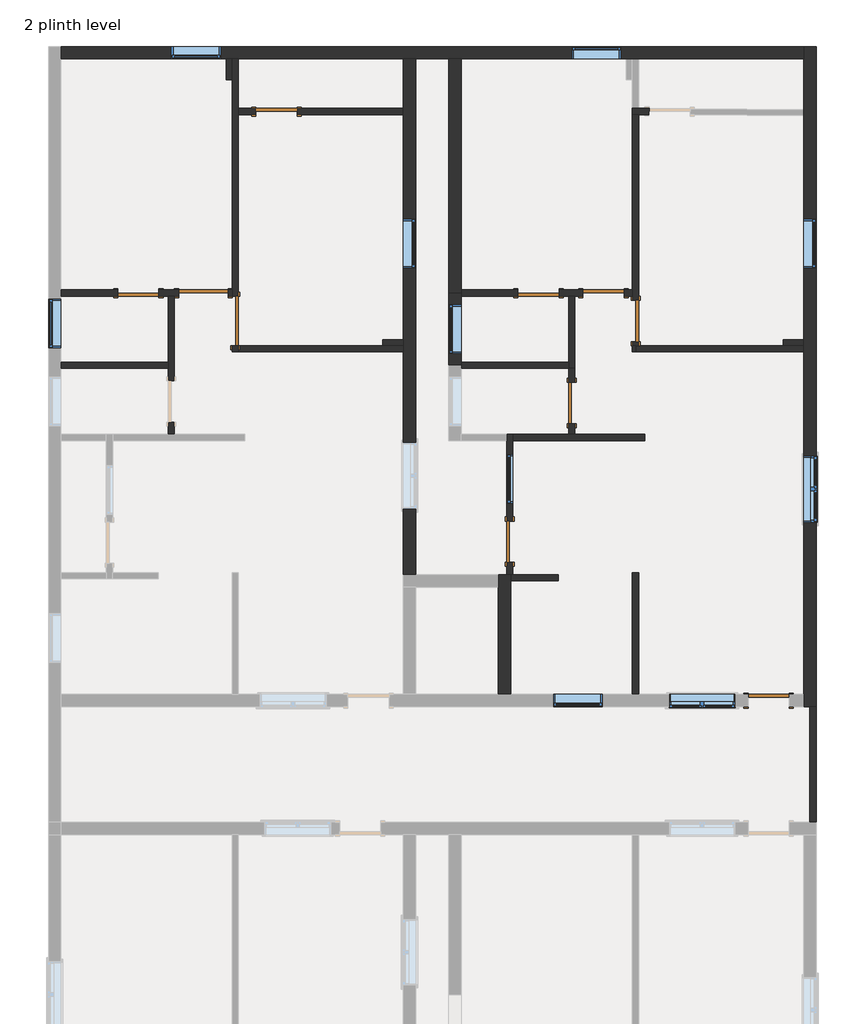
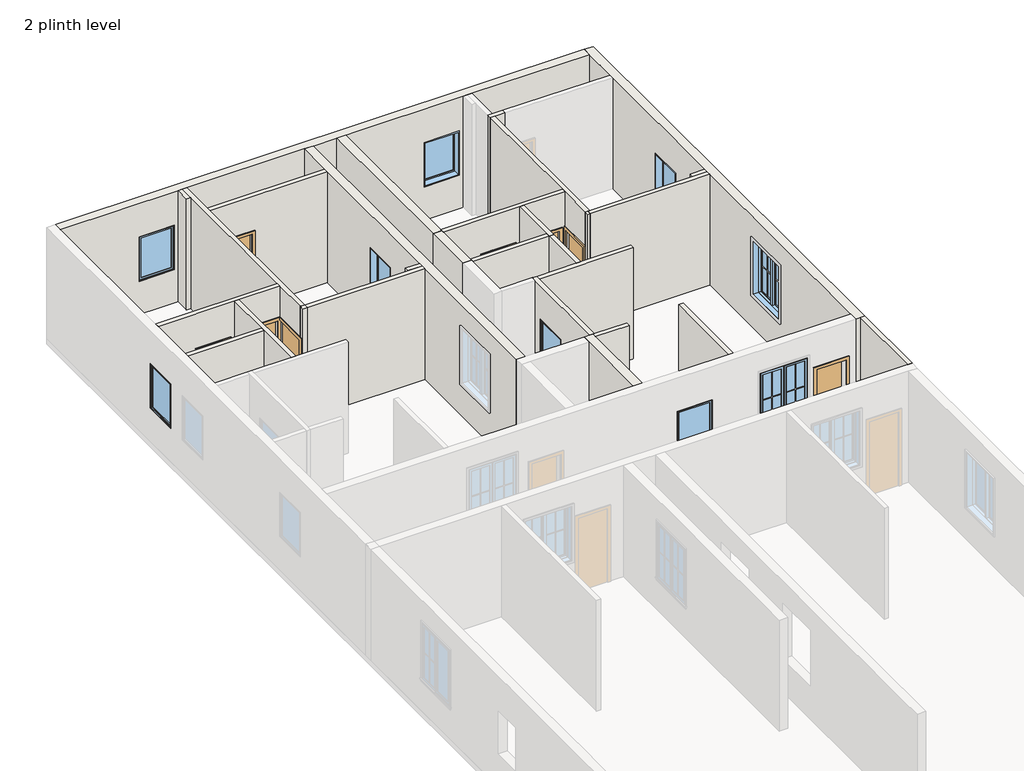
# One storey, part 3 of 4: 29 walls, 10 doors, 10 windows.
"""IFC4 building model written with IfcOpenShell, lengths in millimetres."""

from ifc_helpers import new_model, si_unit, frame, origin, place, context, project, spatial, polyline, outline, extrude, faceted_brep, transform, mapped, element, save
from components import door_d8f5dbb5, door_a1484949, door_f2b275c1, door_e5f9f3c4, window_c1f32544, window_41a96561, window_8377141f

model = new_model("IFC4")

# Units and contexts
model_context = context("Model", 3, world=origin())
ifc_project = project(units=[si_unit("LENGTHUNIT", "METRE", prefix="MILLI")], contexts=[model_context])

# Site, building, storey
site = spatial("IfcSite", under=ifc_project)
building = spatial("IfcBuilding", under=site)
storey = spatial("IfcBuildingStorey", under=building, Name="2 plinth level", Elevation=457.2)

# Doors
placement = place(None, origin())
door_shape = door_d8f5dbb5(model_context)
element("IfcDoor", 1, ObjectType="Single-Flush : 30\" x 80\"", at=placement, inside=storey, context=model_context, shape_type="MappedRepresentation", body=[
    mapped(door_shape, transform((1896.0224532, 9468.2695551, 457.2), x_axis=(1.0, 0.0, 0.0), y_axis=(0.0, 1.0, 0.0), z_axis=(0.0, 0.0, 1.0))),
])
element("IfcDoor", 2, ObjectType="Single-Flush : 30\" x 80\"", at=placement, inside=storey, context=model_context, shape_type="MappedRepresentation", body=[
    mapped(door_shape, transform((2486.5724532, 8953.9195551, 457.2), x_axis=(0.0, -1.0, 0.0), y_axis=(1.0, 0.0, 0.0), z_axis=(0.0, 0.0, 1.0))),
])
door_2_shape = door_a1484949(model_context)
element("IfcDoor", 3, ObjectType="Single-Flush : 30\" x 80\"", at=placement, inside=storey, context=model_context, shape_type="MappedRepresentation", body=[
    mapped(door_2_shape, transform((4944.0224532, 1943.5195552, 457.2), x_axis=(1.0, 0.0, 0.0), y_axis=(0.0, 1.0, 0.0), z_axis=(0.0, 0.0, 1.0))),
])
door_3_shape = door_f2b275c1(model_context)
element("IfcDoor", 4, ObjectType="Single-Flush : 30\" x 80\"", at=placement, inside=storey, context=model_context, shape_type="MappedRepresentation", body=[
    mapped(door_3_shape, transform((162.4724532, 4877.2195551, 457.2), x_axis=(0.0, -1.0, 0.0), y_axis=(1.0, 0.0, 0.0), z_axis=(0.0, 0.0, 1.0))),
])
element("IfcDoor", 5, ObjectType="Single-Flush : 30\" x 80\"", at=placement, inside=storey, context=model_context, shape_type="MappedRepresentation", body=[
    mapped(door_3_shape, transform((1305.4724532, 7439.4445551, 457.2), x_axis=(0.0, -1.0, 0.0), y_axis=(1.0, 0.0, 0.0), z_axis=(0.0, 0.0, 1.0))),
])
element("IfcDoor", 6, ObjectType="Single-Flush : 30\" x 80\"", at=placement, inside=storey, context=model_context, shape_type="MappedRepresentation", body=[
    mapped(door_3_shape, transform((695.8724532, 9468.2695551, 457.2), x_axis=(1.0, 0.0, 0.0), y_axis=(0.0, 1.0, 0.0), z_axis=(0.0, 0.0, 1.0))),
])
element("IfcDoor", 7, ObjectType="Single-Flush : 30\" x 80\"", at=placement, inside=storey, context=model_context, shape_type="MappedRepresentation", body=[
    mapped(door_3_shape, transform((-6695.5275468, 9468.2695551, 457.2), x_axis=(1.0, 0.0, 0.0), y_axis=(0.0, 1.0, 0.0), z_axis=(0.0, 0.0, 1.0))),
])
element("IfcDoor", 8, ObjectType="Single-Flush : 30\" x 80\"", at=placement, inside=storey, context=model_context, shape_type="MappedRepresentation", body=[
    mapped(door_3_shape, transform((-4142.8275468, 12820.5786144, 457.2), x_axis=(-1.0, 0.0, 0.0), y_axis=(0.0, -1.0, 0.0), z_axis=(0.0, 0.0, 1.0))),
])
door_4_shape = door_e5f9f3c4(model_context)
element("IfcDoor", 9, ObjectType="Single-Flush : 36\" x 84\"", at=placement, inside=storey, context=model_context, shape_type="MappedRepresentation", body=[
    mapped(door_4_shape, transform((-5495.3775468, 9468.2695551, 457.2), x_axis=(1.0, 0.0, 0.0), y_axis=(0.0, 1.0, 0.0), z_axis=(0.0, 0.0, 1.0))),
])
element("IfcDoor", 10, ObjectType="Single-Flush : 36\" x 84\"", at=placement, inside=storey, context=model_context, shape_type="MappedRepresentation", body=[
    mapped(door_4_shape, transform((-4904.8275468, 8953.9195551, 457.2), x_axis=(0.0, -1.0, 0.0), y_axis=(1.0, 0.0, 0.0), z_axis=(0.0, 0.0, 1.0))),
])

# Walls
element("IfcWall", 11, ObjectType="4.5\"", at=placement, inside=storey, context=model_context, shape_type="Brep", body=[
    faceted_brep([(-4847.6775468, 13792.6195551, 3505.2), (-4847.6775468, 12877.7286144, 3505.2), (-4847.6775468, 12763.4286144, 3505.2), (-4847.6775468, 8496.7195551, 3505.2), (-4847.6775468, 8496.7195551, 2590.8), (-4847.6775468, 9411.1195551, 2590.8), (-4847.6775468, 9411.1195551, 457.2), (-4847.6775468, 12763.4286144, 457.2), (-4847.6775468, 12877.7286144, 457.2), (-4847.6775468, 13792.6195551, 457.2), (-4961.9775468, 8496.7195551, 3505.2), (-4961.9775468, 9411.1195551, 3505.2), (-4961.9775468, 9525.4195551, 3505.2), (-4961.9775468, 13792.6195551, 3505.2), (-4961.9775468, 13792.6195551, 457.2), (-4961.9775468, 9525.4195551, 457.2), (-4961.9775468, 9411.1195551, 457.2), (-4961.9775468, 9411.1195551, 2590.8), (-4961.9775468, 8496.7195551, 2590.8)], [[[0, 1, 2, 3, 4, 5, 6, 7, 8, 9]], [[10, 11, 12, 13, 14, 15, 16, 17, 18]], [[14, 9, 8, 7, 6, 16, 15]], [[3, 2, 1, 0, 13, 12, 11, 10]], [[0, 9, 14, 13]], [[3, 10, 18, 4]], [[17, 5, 4, 18]], [[5, 17, 16, 6]]]),
])
element("IfcWall", 12, ObjectType="4.5\"", at=placement, inside=storey, context=model_context, shape_type="SweptSolid", body=[
    extrude(outline(polyline([(457.2, -4847.6775468), (457.2, -4523.8275468), (2489.2, -4523.8275468), (2489.2, -3761.8275468), (457.2, -3761.8275468), (457.2, -1799.6775468), (3505.2, -1799.6775468), (3505.2, -4847.6775468), (457.2, -4847.6775468)])), frame((0.0, 12763.4286144, 0.0), z_axis=(0.0, 1.0, 0.0), x_axis=(0.0, 0.0, 1.0)), (0.0, 0.0, 1.0), 114.3),
])
element("IfcWall", 13, ObjectType="4.5\"", at=placement, inside=storey, context=model_context, shape_type="Brep", body=[
    faceted_brep([(-6314.5275468, 9411.1195551, 2489.2), (-6314.5275468, 9411.1195551, 457.2), (-6143.0775468, 9411.1195551, 457.2), (-6028.7775468, 9411.1195551, 457.2), (-5952.5775468, 9411.1195551, 457.2), (-5952.5775468, 9411.1195551, 2590.8), (-5038.1775468, 9411.1195551, 2590.8), (-5038.1775468, 9411.1195551, 457.2), (-4961.9775468, 9411.1195551, 457.2), (-4961.9775468, 9411.1195551, 2590.8), (-4961.9775468, 9411.1195551, 3505.2), (-6028.7775468, 9411.1195551, 3505.2), (-6143.0775468, 9411.1195551, 3505.2), (-8124.2775468, 9411.1195551, 3505.2), (-8124.2775468, 9411.1195551, 457.2), (-7076.5275468, 9411.1195551, 457.2), (-7076.5275468, 9411.1195551, 2489.2), (-5952.5775468, 9525.4195551, 457.2), (-6314.5275468, 9525.4195551, 457.2), (-6314.5275468, 9525.4195551, 2489.2), (-7076.5275468, 9525.4195551, 2489.2), (-7076.5275468, 9525.4195551, 457.2), (-8124.2775468, 9525.4195551, 457.2), (-8124.2775468, 9525.4195551, 3505.2), (-4961.9775468, 9525.4195551, 3505.2), (-4961.9775468, 9525.4195551, 457.2), (-5038.1775468, 9525.4195551, 457.2), (-5038.1775468, 9525.4195551, 2590.8), (-5952.5775468, 9525.4195551, 2590.8)], [[[0, 1, 2, 3, 4, 5, 6, 7, 8, 9, 10, 11, 12, 13, 14, 15, 16]], [[17, 18, 19, 20, 21, 22, 23, 24, 25, 26, 27, 28]], [[8, 7, 26, 25]], [[15, 14, 22, 21]], [[4, 3, 2, 1, 18, 17]], [[13, 12, 11, 10, 24, 23]], [[14, 13, 23, 22]], [[10, 9, 8, 25, 24]], [[27, 26, 7, 6]], [[28, 27, 6, 5]], [[17, 28, 5, 4]], [[19, 18, 1, 0]], [[20, 19, 0, 16]], [[21, 20, 16, 15]]]),
])
element("IfcWall", 14, ObjectType="4.5\"", at=placement, inside=storey, context=model_context, shape_type="SweptSolid", body=[
    extrude(outline(polyline([(-8124.2775468, 8191.9195552), (-6143.0775468, 8191.9195552), (-6143.0775468, 8077.6195552), (-8124.2775468, 8077.6195552), (-8124.2775468, 8191.9195552)])), frame((0.0, 0.0, 457.2), z_axis=(0.0, 0.0, 1.0), x_axis=(1.0, 0.0, 0.0)), (0.0, 0.0, 1.0), 3048.0),
])
element("IfcWall", 15, ObjectType="4.5\"", at=placement, inside=storey, context=model_context, shape_type="Brep", body=[
    faceted_brep([(-6028.7775468, 6858.4195551, 457.2), (-6028.7775468, 7087.0195551, 457.2), (-6028.7775468, 7087.0195551, 2489.2), (-6028.7775468, 7849.0195551, 2489.2), (-6028.7775468, 7849.0195551, 457.2), (-6028.7775468, 9411.1195551, 457.2), (-6028.7775468, 9411.1195551, 3505.2), (-6028.7775468, 6858.4195551, 3505.2), (-6143.0775468, 7087.0195551, 2489.2), (-6143.0775468, 7087.0195551, 457.2), (-6143.0775468, 6858.4195551, 457.2), (-6143.0775468, 6858.4195551, 3505.2), (-6143.0775468, 8077.6195552, 3505.2), (-6143.0775468, 8191.9195552, 3505.2), (-6143.0775468, 9411.1195551, 3505.2), (-6143.0775468, 9411.1195551, 457.2), (-6143.0775468, 8191.9195552, 457.2), (-6143.0775468, 8077.6195552, 457.2), (-6143.0775468, 7849.0195551, 457.2), (-6143.0775468, 7849.0195551, 2489.2)], [[[0, 1, 2, 3, 4, 5, 6, 7]], [[8, 9, 10, 11, 12, 13, 14, 15, 16, 17, 18, 19]], [[10, 9, 1, 0]], [[18, 17, 16, 15, 5, 4]], [[7, 6, 14, 13, 12, 11]], [[6, 5, 15, 14]], [[0, 7, 11, 10]], [[2, 1, 9, 8]], [[3, 2, 8, 19]], [[4, 3, 19, 18]]]),
])
element("IfcWall", 16, ObjectType="4.5\"", at=placement, inside=storey, context=model_context, shape_type="SweptSolid", body=[
    extrude(outline(polyline([(2429.4224532, 2057.8195552), (2429.4224532, 4305.7195551), (2543.7224532, 4305.7195551), (2543.7224532, 2057.8195552), (2429.4224532, 2057.8195552)])), frame((0.0, 0.0, 457.2), z_axis=(0.0, 0.0, 1.0), x_axis=(1.0, 0.0, 0.0)), (0.0, 0.0, 1.0), 3048.0),
])
element("IfcWall", 17, ObjectType="4.5\"", at=placement, inside=storey, context=model_context, shape_type="Brep", body=[
    faceted_brep([(105.3224532, 4496.2195551, 2489.2), (105.3224532, 4496.2195551, 457.2), (105.3224532, 4267.6195551, 457.2), (105.3224532, 4267.6195551, 3505.2), (105.3224532, 6744.1195551, 3505.2), (105.3224532, 6858.4195551, 3505.2), (105.3224532, 6858.4195551, 457.2), (105.3224532, 6744.1195551, 457.2), (105.3224532, 5258.2195551, 457.2), (105.3224532, 5258.2195551, 2489.2), (105.3224532, 6496.4695551, 2590.8), (105.3224532, 5582.0695551, 2590.8), (105.3224532, 5582.0695551, 1371.6), (105.3224532, 6496.4695551, 1371.6), (219.6224532, 4267.6195551, 457.2), (219.6224532, 4496.2195551, 457.2), (219.6224532, 4496.2195551, 2489.2), (219.6224532, 5258.2195551, 2489.2), (219.6224532, 5258.2195551, 457.2), (219.6224532, 6744.1195551, 457.2), (219.6224532, 6858.4195551, 457.2), (219.6224532, 6858.4195551, 3505.2), (219.6224532, 6744.1195551, 3505.2), (219.6224532, 4267.6195551, 3505.2), (219.6224532, 6496.4695551, 2590.8), (219.6224532, 6496.4695551, 1371.6), (219.6224532, 5582.0695551, 1371.6), (219.6224532, 5582.0695551, 2590.8), (181.5224532, 4267.6195551, 457.2), (181.5224532, 4267.6195551, 3505.2)], [[[0, 1, 2, 3, 4, 5, 6, 7, 8, 9], [10, 11, 12, 13]], [[14, 15, 16, 17, 18, 19, 20, 21, 22, 23], [24, 25, 26, 27]], [[2, 1, 15, 14, 28]], [[8, 7, 6, 20, 19, 18]], [[5, 4, 3, 29, 23, 22, 21]], [[6, 5, 21, 20]], [[3, 2, 28, 14, 23, 29]], [[16, 15, 1, 0]], [[17, 16, 0, 9]], [[18, 17, 9, 8]], [[25, 24, 10, 13]], [[26, 25, 13, 12]], [[27, 26, 12, 11]], [[24, 27, 11, 10]]]),
])
element("IfcWall", 18, ObjectType="4.5\"", at=placement, inside=storey, context=model_context, shape_type="Brep", body=[
    faceted_brep([(-4961.9775468, 8382.4195551, 457.2), (-4847.6775468, 8382.4195551, 457.2), (-4847.6775468, 8382.4195551, 3505.2), (-4961.9775468, 8382.4195551, 3505.2), (-4961.9775468, 8496.7195551, 457.2), (-4961.9775468, 8496.7195551, 2590.8), (-4961.9775468, 8496.7195551, 3505.2), (-4847.6775468, 8496.7195551, 3505.2), (-4847.6775468, 8496.7195551, 2590.8), (-4847.6775468, 8496.7195551, 457.2)], [[[0, 1, 2, 3]], [[4, 5, 6, 7, 8, 9]], [[1, 0, 4, 9]], [[3, 2, 7, 6]], [[0, 3, 6, 5, 4]], [[2, 1, 9, 8, 7]]]),
])
element("IfcWall", 19, ObjectType="4.5\"", at=placement, inside=storey, context=model_context, shape_type="Brep", body=[
    faceted_brep([(2543.7224532, 8496.7195551, 457.2), (2543.7224532, 8572.9195551, 457.2), (2543.7224532, 8572.9195551, 2489.2), (2543.7224532, 9334.9195551, 2489.2), (2543.7224532, 9334.9195551, 457.2), (2543.7224532, 12765.2849744, 457.2), (2543.7224532, 12765.2849744, 3505.2), (2543.7224532, 8496.7195551, 3505.2), (2429.4224532, 8572.9195551, 2489.2), (2429.4224532, 8572.9195551, 457.2), (2429.4224532, 8496.7195551, 457.2), (2429.4224532, 8496.7195551, 3505.2), (2429.4224532, 9411.1195551, 3505.2), (2429.4224532, 9525.4195551, 3505.2), (2429.4224532, 12766.2150465, 3505.2), (2429.4224532, 12766.2150465, 457.2), (2429.4224532, 9525.4195551, 457.2), (2429.4224532, 9411.1195551, 457.2), (2429.4224532, 9334.9195551, 457.2), (2429.4224532, 9334.9195551, 2489.2), (2486.5724532, 8496.7195551, 457.2), (2486.5724532, 8496.7195551, 3505.2)], [[[0, 1, 2, 3, 4, 5, 6, 7]], [[8, 9, 10, 11, 12, 13, 14, 15, 16, 17, 18, 19]], [[10, 9, 1, 0, 20]], [[18, 17, 16, 15, 5, 4]], [[7, 6, 14, 13, 12, 11, 21]], [[6, 5, 15, 14]], [[0, 7, 21, 11, 10, 20]], [[2, 1, 9, 8]], [[3, 2, 8, 19]], [[4, 3, 19, 18]]]),
])
element("IfcWall", 20, ObjectType="4.5\"", at=placement, inside=storey, context=model_context, shape_type="Brep", body=[
    faceted_brep([(2429.4224532, 12880.5188304, 3505.2), (2543.7224532, 12879.5887584, 3505.2), (2810.7318517, 12877.4160728, 3505.2), (2810.7318517, 12877.4160728, 2489.2), (2734.5343743, 12878.0361003, 2489.2), (2734.5343743, 12878.0361003, 457.2), (2543.7224532, 12879.5887584, 457.2), (2429.4224532, 12880.5188304, 457.2), (2809.8018105, 12763.1198566, 3505.2), (2543.7224532, 12765.2849744, 3505.2), (2429.4224532, 12766.2150465, 3505.2), (2429.4224532, 12766.2150465, 457.2), (2543.7224532, 12765.2849744, 457.2), (2733.604333, 12763.7398841, 457.2), (2733.604333, 12763.7398841, 2489.2), (2809.8018105, 12763.1198566, 2489.2), (2809.8283078, 12766.376211, 3505.2), (2809.8283078, 12766.376211, 2489.2)], [[[0, 1, 2, 3, 4, 5, 6, 7]], [[8, 9, 10, 11, 12, 13, 14, 15]], [[11, 7, 6, 5, 13, 12]], [[2, 1, 0, 10, 9, 8, 16]], [[2, 16, 8, 15, 17, 3]], [[0, 7, 11, 10]], [[14, 4, 3, 17, 15]], [[4, 14, 13, 5]]]),
])
element("IfcWall", 21, ObjectType="4.5\"", at=placement, inside=storey, context=model_context, shape_type="Brep", body=[
    faceted_brep([(2277.0224532, 9411.1195551, 2489.2), (2277.0224532, 9411.1195551, 457.2), (2429.4224532, 9411.1195551, 457.2), (2429.4224532, 9411.1195551, 3505.2), (1362.6224532, 9411.1195551, 3505.2), (1248.3224532, 9411.1195551, 3505.2), (-732.8775468, 9411.1195551, 3505.2), (-732.8775468, 9411.1195551, 457.2), (314.8724532, 9411.1195551, 457.2), (314.8724532, 9411.1195551, 2489.2), (1076.8724532, 9411.1195551, 2489.2), (1076.8724532, 9411.1195551, 457.2), (1248.3224532, 9411.1195551, 457.2), (1362.6224532, 9411.1195551, 457.2), (1515.0224532, 9411.1195551, 457.2), (1515.0224532, 9411.1195551, 2489.2), (2429.4224532, 9525.4195551, 457.2), (2277.0224532, 9525.4195551, 457.2), (2277.0224532, 9525.4195551, 2489.2), (1515.0224532, 9525.4195551, 2489.2), (1515.0224532, 9525.4195551, 457.2), (1076.8724532, 9525.4195551, 457.2), (1076.8724532, 9525.4195551, 2489.2), (314.8724532, 9525.4195551, 2489.2), (314.8724532, 9525.4195551, 457.2), (-732.8775468, 9525.4195551, 457.2), (-732.8775468, 9525.4195551, 3505.2), (2429.4224532, 9525.4195551, 3505.2), (-732.8775468, 9468.2695551, 457.2), (-732.8775468, 9468.2695551, 3505.2)], [[[0, 1, 2, 3, 4, 5, 6, 7, 8, 9, 10, 11, 12, 13, 14, 15]], [[16, 17, 18, 19, 20, 21, 22, 23, 24, 25, 26, 27]], [[8, 7, 28, 25, 24]], [[2, 1, 17, 16]], [[14, 13, 12, 11, 21, 20]], [[6, 5, 4, 3, 27, 26, 29]], [[7, 6, 29, 26, 25, 28]], [[3, 2, 16, 27]], [[22, 21, 11, 10]], [[23, 22, 10, 9]], [[24, 23, 9, 8]], [[18, 17, 1, 0]], [[19, 18, 0, 15]], [[20, 19, 15, 14]]]),
])
element("IfcWall", 22, ObjectType="4.5\"", at=placement, inside=storey, context=model_context, shape_type="Brep", body=[
    faceted_brep([(1248.3224532, 9411.1195551, 457.2), (1248.3224532, 8191.9195551, 457.2), (1248.3224532, 8077.6195551, 457.2), (1248.3224532, 8077.6195551, 3505.2), (1248.3224532, 8191.9195551, 3505.2), (1248.3224532, 9411.1195551, 3505.2), (1362.6224532, 9411.1195551, 457.2), (1362.6224532, 9411.1195551, 3505.2), (1362.6224532, 8077.6195551, 3505.2), (1362.6224532, 8077.6195551, 457.2)], [[[0, 1, 2, 3, 4, 5]], [[6, 7, 8, 9]], [[2, 1, 0, 6, 9]], [[5, 4, 3, 8, 7]], [[3, 2, 9, 8]], [[0, 5, 7, 6]]]),
])
element("IfcWall", 23, ObjectType="4.5\"", at=placement, inside=storey, context=model_context, shape_type="Brep", body=[
    faceted_brep([(-732.8775468, 8077.6195551, 457.2), (1248.3224532, 8077.6195551, 457.2), (1248.3224532, 8077.6195551, 3505.2), (-732.8775468, 8077.6195551, 3505.2), (-732.8775468, 8191.9195551, 457.2), (-732.8775468, 8191.9195551, 3505.2), (1248.3224532, 8191.9195551, 3505.2), (1248.3224532, 8191.9195551, 457.2), (-732.8775468, 8134.7695551, 457.2), (-732.8775468, 8134.7695551, 3505.2)], [[[0, 1, 2, 3]], [[4, 5, 6, 7]], [[1, 0, 8, 4, 7]], [[3, 2, 6, 5, 9]], [[0, 3, 9, 5, 4, 8]], [[2, 1, 7, 6]]]),
])
element("IfcWall", 24, ObjectType="4.5\"", at=placement, inside=storey, context=model_context, shape_type="Brep", body=[
    faceted_brep([(219.6224532, 6744.1195551, 457.2), (2658.0224532, 6744.1195551, 457.2), (2658.0224532, 6744.1195551, 3505.2), (219.6224532, 6744.1195551, 3505.2), (219.6224532, 6858.4195551, 457.2), (219.6224532, 6858.4195551, 3505.2), (1248.3224532, 6858.4195551, 3505.2), (1362.6224532, 6858.4195551, 3505.2), (2658.0224532, 6858.4195551, 3505.2), (2658.0224532, 6858.4195551, 457.2), (1362.6224532, 6858.4195551, 457.2), (1248.3224532, 6858.4195551, 457.2)], [[[0, 1, 2, 3]], [[4, 5, 6, 7, 8, 9, 10, 11]], [[1, 0, 4, 11, 10, 9]], [[2, 1, 9, 8]], [[3, 2, 8, 7, 6, 5]], [[0, 3, 5, 4]]]),
])
element("IfcWall", 25, ObjectType="4.5\"", at=placement, inside=storey, context=model_context, shape_type="SweptSolid", body=[
    extrude(outline(polyline([(2486.5724532, 8382.4195551), (2429.4224532, 8382.4195551), (2429.4224532, 8496.7195551), (2486.5724532, 8496.7195551), (2486.5724532, 8382.4195551)])), frame((0.0, 0.0, 457.2), z_axis=(0.0, 0.0, 1.0), x_axis=(1.0, 0.0, 0.0)), (0.0, 0.0, 1.0), 3048.0),
])
element("IfcWall", 26, ObjectType="4.5\"", at=placement, inside=storey, context=model_context, shape_type="Brep", body=[
    faceted_brep([(1058.8844648, 4267.6195551, 457.2), (219.6224532, 4267.6195551, 457.2), (181.5224532, 4267.6195551, 457.2), (181.5224532, 4267.6195551, 3505.2), (219.6224532, 4267.6195551, 3505.2), (1058.8844648, 4267.6195551, 3505.2), (1058.8844648, 4153.3195551, 457.2), (1058.8844648, 4153.3195551, 3505.2), (181.5224532, 4153.3195551, 3505.2), (181.5224532, 4153.3195551, 457.2)], [[[0, 1, 2, 3, 4, 5]], [[6, 7, 8, 9]], [[2, 1, 0, 6, 9]], [[5, 4, 3, 8, 7]], [[0, 5, 7, 6]], [[3, 2, 9, 8]]]),
])
element("IfcWall", 27, ObjectType="4.5\"", at=placement, inside=storey, context=model_context, shape_type="SweptSolid", body=[
    extrude(outline(polyline([(-1799.6775468, 8382.4195551), (-4847.6775468, 8382.4195551), (-4847.6775468, 8496.7195551), (-1799.6775468, 8496.7195551), (-1799.6775468, 8382.4195551)])), frame((0.0, 0.0, 457.2), z_axis=(0.0, 0.0, 1.0), x_axis=(1.0, 0.0, 0.0)), (0.0, 0.0, 1.0), 3048.0),
])
element("IfcWall", 28, ObjectType="4.5\"", at=placement, inside=storey, context=model_context, shape_type="SweptSolid", body=[
    extrude(outline(polyline([(7058.4445551, 2489.2), (7058.4445551, 457.2), (6858.4195551, 457.2), (6858.4195551, 3505.2), (8077.6195551, 3505.2), (8077.6195551, 457.2), (7820.4445551, 457.2), (7820.4445551, 2489.2), (7058.4445551, 2489.2)])), frame((1248.3224532, 0.0, 0.0), z_axis=(1.0, 0.0, 0.0), x_axis=(0.0, 1.0, 0.0)), (0.0, 0.0, 1.0), 114.3),
])
element("IfcWall", 29, ObjectType="4.5\"", at=placement, inside=storey, context=model_context, shape_type="SweptSolid", body=[
    extrude(outline(polyline([(5820.3224532, 1829.2195552), (5820.3224532, -304.3804449), (5706.0224532, -304.3804449), (5706.0224532, 1829.2195552), (5820.3224532, 1829.2195552)])), frame((0.0, 0.0, 457.2), z_axis=(0.0, 0.0, 1.0), x_axis=(1.0, 0.0, 0.0)), (0.0, 0.0, 1.0), 3048.0),
])
element("IfcWall", 30, ObjectType="4.5\"", at=placement, inside=storey, context=model_context, shape_type="Brep", body=[
    faceted_brep([(2486.5724532, 8382.4195551, 457.2), (5591.7224532, 8382.4195551, 457.2), (5591.7224532, 8382.4195551, 3505.2), (2486.5724532, 8382.4195551, 3505.2), (2486.5724532, 8496.7195551, 457.2), (2486.5724532, 8496.7195551, 3505.2), (2543.7224532, 8496.7195551, 3505.2), (5591.7224532, 8496.7195551, 3505.2), (5591.7224532, 8496.7195551, 457.2), (2543.7224532, 8496.7195551, 457.2)], [[[0, 1, 2, 3]], [[4, 5, 6, 7, 8, 9]], [[1, 0, 4, 9, 8]], [[3, 2, 7, 6, 5]], [[0, 3, 5, 4]], [[2, 1, 8, 7]]]),
])
element("IfcWall", 31, ObjectType="4.5\"", at=placement, inside=storey, context=model_context, shape_type="SweptSolid", body=[
    extrude(outline(polyline([(-2180.6775468, 8611.0195551), (-1799.6775468, 8611.0195551), (-1799.6775468, 8496.7195551), (-2180.6775468, 8496.7195551), (-2180.6775468, 8611.0195551)])), frame((0.0, 0.0, 457.2), z_axis=(0.0, 0.0, 1.0), x_axis=(1.0, 0.0, 0.0)), (0.0, 0.0, 1.0), 3048.0),
])
element("IfcWall", 32, ObjectType="4.5\"", at=placement, inside=storey, context=model_context, shape_type="SweptSolid", body=[
    extrude(outline(polyline([(-5076.2775468, 13411.6195551), (-5076.2775468, 13792.6195551), (-4961.9775468, 13792.6195551), (-4961.9775468, 13411.6195551), (-5076.2775468, 13411.6195551)])), frame((0.0, 0.0, 457.2), z_axis=(0.0, 0.0, 1.0), x_axis=(1.0, 0.0, 0.0)), (0.0, 0.0, 1.0), 3048.0),
])
element("IfcWall", 33, ObjectType="4.5\"", at=placement, inside=storey, context=model_context, shape_type="SweptSolid", body=[
    extrude(outline(polyline([(5210.7224532, 8611.0195551), (5591.7224532, 8611.0195551), (5591.7224532, 8496.7195551), (5210.7224532, 8496.7195551), (5210.7224532, 8611.0195551)])), frame((0.0, 0.0, 457.2), z_axis=(0.0, 0.0, 1.0), x_axis=(1.0, 0.0, 0.0)), (0.0, 0.0, 1.0), 3048.0),
])
element("IfcWall", 34, ObjectType="9\"", at=placement, inside=storey, context=model_context, shape_type="Brep", body=[
    faceted_brep([(5591.7224532, 14021.2195551, 457.2), (5591.7224532, 13792.6195551, 457.2), (5591.7224532, 12858.0434078, 457.2), (5591.7224532, 12743.7396238, 457.2), (5591.7224532, 8611.0195551, 457.2), (5591.7224532, 8496.7195551, 457.2), (5591.7224532, 8382.4195551, 457.2), (5591.7224532, 2057.8195552, 457.2), (5591.7224532, 1829.2195552, 457.2), (5591.7224532, 1829.2195552, 3505.2), (5591.7224532, 2057.8195552, 3505.2), (5591.7224532, 8382.4195551, 3505.2), (5591.7224532, 8496.7195551, 3505.2), (5591.7224532, 8611.0195551, 3505.2), (5591.7224532, 12743.7396238, 3505.2), (5591.7224532, 12858.0434078, 3505.2), (5591.7224532, 13792.6195551, 3505.2), (5591.7224532, 14021.2195551, 3505.2), (5591.7224532, 9925.4695551, 2590.8), (5591.7224532, 9925.4695551, 1371.6), (5591.7224532, 10839.8695551, 1371.6), (5591.7224532, 10839.8695551, 2590.8), (5591.7224532, 5239.1695551, 2895.6), (5591.7224532, 5239.1695551, 1371.6), (5591.7224532, 6458.3695551, 1371.6), (5591.7224532, 6458.3695551, 2895.6), (5820.3224532, 14021.2195551, 457.2), (5820.3224532, 14021.2195551, 3505.2), (5820.3224532, 1829.2195552, 3505.2), (5820.3224532, 1829.2195552, 457.2), (5820.3224532, 9925.4695551, 2590.8), (5820.3224532, 10839.8695551, 2590.8), (5820.3224532, 10839.8695551, 1371.6), (5820.3224532, 9925.4695551, 1371.6), (5820.3224532, 5239.1695551, 2895.6), (5820.3224532, 6458.3695551, 2895.6), (5820.3224532, 6458.3695551, 1371.6), (5820.3224532, 5239.1695551, 1371.6), (5706.0224532, 1829.2195552, 457.2), (5706.0224532, 1829.2195552, 3505.2)], [[[0, 1, 2, 3, 4, 5, 6, 7, 8, 9, 10, 11, 12, 13, 14, 15, 16, 17], [18, 19, 20, 21], [22, 23, 24, 25]], [[26, 27, 28, 29], [30, 31, 32, 33], [34, 35, 36, 37]], [[8, 7, 6, 5, 4, 3, 2, 1, 0, 26, 29, 38]], [[17, 16, 15, 14, 13, 12, 11, 10, 9, 39, 28, 27]], [[0, 17, 27, 26]], [[9, 8, 38, 29, 28, 39]], [[19, 18, 30, 33]], [[20, 19, 33, 32]], [[21, 20, 32, 31]], [[18, 21, 31, 30]], [[23, 22, 34, 37]], [[24, 23, 37, 36]], [[25, 24, 36, 35]], [[22, 25, 35, 34]]]),
])
element("IfcWall", 35, ObjectType="9\"", at=placement, inside=storey, context=model_context, shape_type="Brep", body=[
    faceted_brep([(5591.7224532, 14021.2195551, 457.2), (-8124.2775468, 14021.2195551, 457.2), (-8124.2775468, 14021.2195551, 3505.2), (5591.7224532, 14021.2195551, 3505.2), (-6085.9275468, 14021.2195551, 2590.8), (-6085.9275468, 14021.2195551, 1371.6), (-5171.5275468, 14021.2195551, 1371.6), (-5171.5275468, 14021.2195551, 2590.8), (2219.8724532, 14021.2195551, 2590.8), (1305.4724532, 14021.2195551, 2590.8), (1305.4724532, 14021.2195551, 1371.6), (2219.8724532, 14021.2195551, 1371.6), (5591.7224532, 13792.6195551, 457.2), (5591.7224532, 13792.6195551, 3505.2), (2543.7224532, 13792.6195551, 3505.2), (2429.4224532, 13792.6195551, 3505.2), (2315.1224532, 13792.6195551, 3505.2), (-732.8775468, 13792.6195551, 3505.2), (-961.4775468, 13792.6195551, 3505.2), (-1571.0775468, 13792.6195551, 3505.2), (-1799.6775468, 13792.6195551, 3505.2), (-4847.6775468, 13792.6195551, 3505.2), (-4961.9775468, 13792.6195551, 3505.2), (-5076.2775468, 13792.6195551, 3505.2), (-8124.2775468, 13792.6195551, 3505.2), (-8124.2775468, 13792.6195551, 457.2), (-5076.2775468, 13792.6195551, 457.2), (-4961.9775468, 13792.6195551, 457.2), (-4847.6775468, 13792.6195551, 457.2), (-1799.6775468, 13792.6195551, 457.2), (-1571.0775468, 13792.6195551, 457.2), (-961.4775468, 13792.6195551, 457.2), (-732.8775468, 13792.6195551, 457.2), (2315.1224532, 13792.6195551, 457.2), (2429.4224532, 13792.6195551, 457.2), (2543.7224532, 13792.6195551, 457.2), (-6085.9275468, 13792.6195551, 2590.8), (-5171.5275468, 13792.6195551, 2590.8), (-5171.5275468, 13792.6195551, 1371.6), (-6085.9275468, 13792.6195551, 1371.6), (2219.8724532, 13792.6195551, 2590.8), (2219.8724532, 13792.6195551, 1371.6), (1305.4724532, 13792.6195551, 1371.6), (1305.4724532, 13792.6195551, 2590.8)], [[[0, 1, 2, 3], [4, 5, 6, 7], [8, 9, 10, 11]], [[12, 13, 14, 15, 16, 17, 18, 19, 20, 21, 22, 23, 24, 25, 26, 27, 28, 29, 30, 31, 32, 33, 34, 35], [36, 37, 38, 39], [40, 41, 42, 43]], [[1, 0, 12, 35, 34, 33, 32, 31, 30, 29, 28, 27, 26, 25]], [[3, 2, 24, 23, 22, 21, 20, 19, 18, 17, 16, 15, 14, 13]], [[2, 1, 25, 24]], [[0, 3, 13, 12]], [[5, 4, 36, 39]], [[6, 5, 39, 38]], [[7, 6, 38, 37]], [[4, 7, 37, 36]], [[41, 40, 8, 11]], [[42, 41, 11, 10]], [[43, 42, 10, 9]], [[40, 43, 9, 8]]]),
])
element("IfcWall", 36, ObjectType="9\"", at=placement, inside=storey, context=model_context, shape_type="Brep", body=[
    faceted_brep([(-961.4775468, 13792.6195551, 457.2), (-961.4775468, 9468.2695551, 457.2), (-961.4775468, 9468.2695551, 3505.2), (-961.4775468, 13792.6195551, 3505.2), (-732.8775468, 13792.6195551, 457.2), (-732.8775468, 13792.6195551, 3505.2), (-732.8775468, 9525.4195551, 3505.2), (-732.8775468, 9468.2695551, 3505.2), (-732.8775468, 9468.2695551, 457.2), (-732.8775468, 9525.4195551, 457.2)], [[[0, 1, 2, 3]], [[4, 5, 6, 7, 8, 9]], [[1, 0, 4, 9, 8]], [[2, 1, 8, 7]], [[3, 2, 7, 6, 5]], [[0, 3, 5, 4]]]),
])
element("IfcWall", 37, ObjectType="9\"", at=placement, inside=storey, context=model_context, shape_type="Brep", body=[
    faceted_brep([(-47.0775468, 4267.6195551, 457.2), (-47.0775468, 4039.0195551, 457.2), (-47.0775468, 2057.8195552, 457.2), (-47.0775468, 2057.8195552, 3505.2), (-47.0775468, 4039.0195551, 3505.2), (-47.0775468, 4267.6195551, 3505.2), (181.5224532, 4267.6195551, 457.2), (181.5224532, 4267.6195551, 3505.2), (181.5224532, 4153.3195551, 3505.2), (181.5224532, 2057.8195552, 3505.2), (181.5224532, 2057.8195552, 457.2), (181.5224532, 4153.3195551, 457.2), (105.3224532, 4267.6195551, 457.2), (105.3224532, 4267.6195551, 3505.2)], [[[0, 1, 2, 3, 4, 5]], [[6, 7, 8, 9, 10, 11]], [[2, 1, 0, 12, 6, 11, 10]], [[5, 4, 3, 9, 8, 7, 13]], [[3, 2, 10, 9]], [[0, 5, 13, 7, 6, 12]]]),
])
element("IfcWall", 38, ObjectType="9\"", at=placement, inside=storey, context=model_context, shape_type="Brep", body=[
    faceted_brep([(-1799.6775468, 13792.6195551, 457.2), (-1799.6775468, 12877.7286144, 457.2), (-1799.6775468, 12763.4286144, 457.2), (-1799.6775468, 8611.0195551, 457.2), (-1799.6775468, 8496.7195551, 457.2), (-1799.6775468, 8382.4195551, 457.2), (-1799.6775468, 4267.6195551, 457.2), (-1799.6775468, 4267.6195551, 3505.2), (-1799.6775468, 8382.4195551, 3505.2), (-1799.6775468, 8496.7195551, 3505.2), (-1799.6775468, 8611.0195551, 3505.2), (-1799.6775468, 12763.4286144, 3505.2), (-1799.6775468, 12877.7286144, 3505.2), (-1799.6775468, 13792.6195551, 3505.2), (-1799.6775468, 9925.4695551, 2590.8), (-1799.6775468, 9925.4695551, 1371.6), (-1799.6775468, 10839.8695551, 1371.6), (-1799.6775468, 10839.8695551, 2590.8), (-1799.6775468, 5486.8195551, 2895.6), (-1799.6775468, 5486.8195551, 1371.6), (-1799.6775468, 6706.0195551, 1371.6), (-1799.6775468, 6706.0195551, 2895.6), (-1571.0775468, 13792.6195551, 457.2), (-1571.0775468, 13792.6195551, 3505.2), (-1571.0775468, 4267.6195551, 3505.2), (-1571.0775468, 4267.6195551, 457.2), (-1571.0775468, 9925.4695551, 2590.8), (-1571.0775468, 10839.8695551, 2590.8), (-1571.0775468, 10839.8695551, 1371.6), (-1571.0775468, 9925.4695551, 1371.6), (-1571.0775468, 5486.8195551, 2895.6), (-1571.0775468, 6706.0195551, 2895.6), (-1571.0775468, 6706.0195551, 1371.6), (-1571.0775468, 5486.8195551, 1371.6)], [[[0, 1, 2, 3, 4, 5, 6, 7, 8, 9, 10, 11, 12, 13], [14, 15, 16, 17], [18, 19, 20, 21]], [[22, 23, 24, 25], [26, 27, 28, 29], [30, 31, 32, 33]], [[6, 5, 4, 3, 2, 1, 0, 22, 25]], [[13, 12, 11, 10, 9, 8, 7, 24, 23]], [[7, 6, 25, 24]], [[0, 13, 23, 22]], [[15, 14, 26, 29]], [[16, 15, 29, 28]], [[17, 16, 28, 27]], [[14, 17, 27, 26]], [[19, 18, 30, 33]], [[20, 19, 33, 32]], [[21, 20, 32, 31]], [[18, 21, 31, 30]]]),
])
element("IfcWall", 39, ObjectType="9\"", at=placement, inside=storey, context=model_context, shape_type="Brep", body=[
    faceted_brep([(-961.4775468, 9468.2695551, 457.2), (-961.4775468, 8134.7695551, 457.2), (-961.4775468, 8134.7695551, 3505.2), (-961.4775468, 9468.2695551, 3505.2), (-961.4775468, 9258.7195551, 2590.8), (-961.4775468, 8344.3195551, 2590.8), (-961.4775468, 8344.3195551, 1371.6), (-961.4775468, 9258.7195551, 1371.6), (-732.8775468, 9468.2695551, 457.2), (-732.8775468, 9468.2695551, 3505.2), (-732.8775468, 9411.1195551, 3505.2), (-732.8775468, 8191.9195551, 3505.2), (-732.8775468, 8134.7695551, 3505.2), (-732.8775468, 8134.7695551, 457.2), (-732.8775468, 8191.9195551, 457.2), (-732.8775468, 9411.1195551, 457.2), (-732.8775468, 9258.7195551, 2590.8), (-732.8775468, 9258.7195551, 1371.6), (-732.8775468, 8344.3195551, 1371.6), (-732.8775468, 8344.3195551, 2590.8)], [[[0, 1, 2, 3], [4, 5, 6, 7]], [[8, 9, 10, 11, 12, 13, 14, 15], [16, 17, 18, 19]], [[1, 0, 8, 15, 14, 13]], [[2, 1, 13, 12]], [[3, 2, 12, 11, 10, 9]], [[0, 3, 9, 8]], [[17, 16, 4, 7]], [[18, 17, 7, 6]], [[19, 18, 6, 5]], [[16, 19, 5, 4]]]),
])

# Windows
window_shape = window_c1f32544(model_context)
element("IfcWindow", 40, ObjectType="Fixed : 36\" x 48\"", at=placement, inside=storey, context=model_context, shape_type="MappedRepresentation", body=[
    mapped(window_shape, transform((-8238.5775468, 8947.5695551, 457.2), x_axis=(0.0, 1.0, 0.0), y_axis=(-1.0, 0.0, 0.0), z_axis=(0.0, 0.0, 1.0))),
])
element("IfcWindow", 41, ObjectType="Fixed : 36\" x 48\"", at=placement, inside=storey, context=model_context, shape_type="MappedRepresentation", body=[
    mapped(window_shape, transform((-5666.8275468, 13906.9195551, 457.2), x_axis=(-1.0, 0.0, 0.0), y_axis=(0.0, -1.0, 0.0), z_axis=(0.0, 0.0, 1.0))),
])
element("IfcWindow", 42, ObjectType="Fixed : 36\" x 48\"", at=placement, inside=storey, context=model_context, shape_type="MappedRepresentation", body=[
    mapped(window_shape, transform((1800.7724532, 13906.9195551, 457.2), x_axis=(1.0, 0.0, 0.0), y_axis=(0.0, 1.0, 0.0), z_axis=(0.0, 0.0, 1.0))),
])
element("IfcWindow", 43, ObjectType="Fixed : 36\" x 48\"", at=placement, inside=storey, context=model_context, shape_type="MappedRepresentation", body=[
    mapped(window_shape, transform((5706.0224532, 10344.5695551, 457.2), x_axis=(0.0, -1.0, 0.0), y_axis=(1.0, 0.0, 0.0), z_axis=(0.0, 0.0, 1.0))),
])
element("IfcWindow", 44, ObjectType="Fixed : 36\" x 48\"", at=placement, inside=storey, context=model_context, shape_type="MappedRepresentation", body=[
    mapped(window_shape, transform((-1685.3775468, 10344.5695551, 457.2), x_axis=(0.0, -1.0, 0.0), y_axis=(1.0, 0.0, 0.0), z_axis=(0.0, 0.0, 1.0))),
])
element("IfcWindow", 45, ObjectType="Fixed : 36\" x 48\"", at=placement, inside=storey, context=model_context, shape_type="MappedRepresentation", body=[
    mapped(window_shape, transform((-847.1775468, 8839.6195551, 457.2), x_axis=(0.0, 1.0, 0.0), y_axis=(-1.0, 0.0, 0.0), z_axis=(0.0, 0.0, 1.0))),
])
element("IfcWindow", 46, ObjectType="Fixed : 36\" x 48\"", at=placement, inside=storey, context=model_context, shape_type="MappedRepresentation", body=[
    mapped(window_shape, transform((1381.6724532, 1943.5195552, 457.2), x_axis=(-1.0, 0.0, 0.0), y_axis=(0.0, -1.0, 0.0), z_axis=(0.0, 0.0, 1.0))),
])
window_2_shape = window_41a96561(model_context)
element("IfcWindow", 47, ObjectType="Fixed : 36\" x 48\"", at=placement, inside=storey, context=model_context, shape_type="MappedRepresentation", body=[
    mapped(window_2_shape, transform((162.4724532, 6077.3695551, 457.2), x_axis=(0.0, 1.0, 0.0), y_axis=(-1.0, 0.0, 0.0), z_axis=(0.0, 0.0, 1.0))),
])
window_3_shape = window_8377141f(model_context)
element("IfcWindow", 48, ObjectType="Window-Casement-Double : 48\" x 60\"", at=placement, inside=storey, context=model_context, shape_type="MappedRepresentation", body=[
    mapped(window_3_shape, transform((3715.2974532, 1943.5195552, 457.2), x_axis=(-1.0, 0.0, 0.0), y_axis=(0.0, -1.0, 0.0), z_axis=(0.0, 0.0, 1.0))),
])
element("IfcWindow", 49, ObjectType="Window-Casement-Double : 48\" x 60\"", at=placement, inside=storey, context=model_context, shape_type="MappedRepresentation", body=[
    mapped(window_3_shape, transform((5706.0224532, 5848.7695551, 457.2), x_axis=(0.0, -1.0, 0.0), y_axis=(1.0, 0.0, 0.0), z_axis=(0.0, 0.0, 1.0))),
])

save(model, "model.ifc")

# Revit data of these elements
# Type "Single-Flush : 30\" x 80\""
#   Type Mark = "5"
#   Construction Type Id = "MDOOR"
#   Assembly Code = "C1020"
#   Analytic Construction = "Metal"
#   Thickness = 0' - 2"
#   Heat Transfer Coefficient (U) = 0.651978 BTU/(h·ft²·°F)
#   Height = 6' - 8"
#   Trim Projection Ext = 0' - 1"
#   Trim Projection Int = 0' - 1"
#   Trim Width = 0' - 3"
#   Width = 2' - 6"
#   Define Thermal Properties by = 1
#   Define Thermal Properties by = 1
#   Door Material = Door - Panel
#   Frame Material = Door - Frame
#   Visual Light Transmittance = 0
#   Solar Heat Gain Coefficient = 0
#   Function = (empty or 0)
#   Wall Closure = (empty or 0)
# Type "Single-Flush : 36\" x 84\""
#   Type Mark = "1"
#   Construction Type Id = "MDOOR"
#   Assembly Code = "C1020"
#   Analytic Construction = "Metal"
#   Thickness = 0' - 2"
#   Heat Transfer Coefficient (U) = 0.651978 BTU/(h·ft²·°F)
#   Height = 7' - 0"
#   Trim Projection Ext = 0' - 1"
#   Trim Projection Int = 0' - 1"
#   Trim Width = 0' - 3"
#   Width = 3' - 0"
#   Define Thermal Properties by = 1
#   Define Thermal Properties by = 1
#   Door Material = Door - Panel
#   Frame Material = Door - Frame
#   Visual Light Transmittance = 0
#   Solar Heat Gain Coefficient = 0
#   Function = (empty or 0)
#   Wall Closure = (empty or 0)
# Type "4.5\""
#   Assembly Code = "B2010"
#   Layers, outside or top first: 0' - 4 1/2" no material (function 1)
# Type "9\""
#   Assembly Code = "B2010"
#   Layers, outside or top first: 0' - 9" no material (function 1)
# Type "Fixed : 36\" x 48\""
#   Type Mark = "1"
#   Construction Type Id = "GSP4R"
#   Assembly Code = "B2020100"
#   Analytic Construction = "1/8 in Pilkington single glazing"
#   Visual Light Transmittance = 0.9
#   Solar Heat Gain Coefficient = 0.78
#   Heat Transfer Coefficient (U) = 0.6496 BTU/(h·ft²·°F)
#   Height = 4' - 0"
#   Default Sill Height = 3' - 0"
#   Width = 3' - 0"
#   Window Inset = 0' - 0 3/4"
#   Define Thermal Properties by = 1
#   Define Thermal Properties by = 1
#   Glass Pane Material = Glass
#   Sash Material = Sash
#   Wall Closure = (empty or 0)
# Type "Window-Casement-Double : 48\" x 60\""
#   Type Mark = "16"
#   Fire Rating = "0.5h"
#   Assembly Code = "B2020100"
#   Analytic Construction = "Double glazing - domestic"
#   Frame Extension [instance default] = 0' - 0 1/4"
#   Window Inset [instance default] = 0' - 0"
#   Wall Thickness [instance default] = 0' - 6"
#   Interior Wall Closure [instance default] = 0' - 2 1/4"
#   Half Width = 2' - 0"
#   Visual Light Transmittance = 0.81
#   Thermal Resistance (R) = 1.8146 (h·ft²·°F)/BTU
#   Solar Heat Gain Coefficient = 0.76
#   Rough Width = 4' - 0 1/2"
#   Rough Height = 5' - 0 1/2"
#   Height = 5' - 0"
#   Heat Transfer Coefficient (U) = 0.5511 BTU/(h·ft²·°F)
#   Exterior Wall Closure [instance default] = 0' - 1 1/4"
#   Extension Jamb [instance default] = 0' - 2 1/4"
#   Default Sill Height = 3' - 0"
#   Width = 4' - 0"
#   Define Thermal Properties by = 0
#   Muntin Visibility = yes
#   Interior Trim Visibility [instance default] = yes
#   Exterior Trim Visibility [instance default] = yes
#   Extension Jamb Visibility [instance default] = yes
#   Interior Trim Material = Wood - Stained
#   Muntin Pattern = Muntin Pattern_2x2 : Muntin Pattern_2x2
#   Interior Trim = Trim-Window-Interior-Flat : Picture Frame
#   Interior Frame Material = Wood - Stained
#   Glass Panel Material = Glass
#   Exterior Trim Material = Clad - White
#   Exterior Trim = Trim-Window-Exterior-Flat : with Sill
#   Exterior Frame Material = Clad - White
#   Wall Closure = (empty or 0)
# Elements 1, 2, 3, 4, 5, 6, 7, 8 (IfcDoor, "Single-Flush : 30\" x 80\"")
#   Phase Created = New Construction
#   Materials on its faces: "Door - Frame", "Door - Panel"
# Elements 9, 10 (IfcDoor, "Single-Flush : 36\" x 84\"")
#   Phase Created = New Construction
#   Materials on its faces: "Door - Frame", "Door - Panel"
# Elements 11, 12, 13, 14, 15, 16, 17, 18, 19, 20, 21, 22, 23, 24, 25, 26, 27, 28, 29, 30, 31, 32, 33 (IfcWall, "4.5\"")
#   Top Offset = 0' - 0"
#   Base Offset = 0' - 0"
#   wall height = 10' - 0"
#   Phase Created = New Construction
#   Base Constraint = 2 plinth level
#   Top Constraint = 3 wall level
#   Materials on its faces: "Default Wall"
# Elements 34, 35, 36, 37, 38, 39 (IfcWall, "9\"")
#   Top Offset = 0' - 0"
#   Base Offset = 0' - 0"
#   wall height = 10' - 0"
#   Phase Created = New Construction
#   Base Constraint = 2 plinth level
#   Top Constraint = 3 wall level
#   Materials on its faces: "Default Wall"
# Element 40 (IfcWindow, "Fixed : 36\" x 48\"")
#   Mark = "9"
#   Phase Created = New Construction
#   Materials on its faces: "Sash", "Glass"
# Element 41 (IfcWindow, "Fixed : 36\" x 48\"")
#   Mark = "10"
#   Phase Created = New Construction
#   Materials on its faces: "Sash", "Glass"
# Element 42 (IfcWindow, "Fixed : 36\" x 48\"")
#   Mark = "11"
#   Phase Created = New Construction
#   Materials on its faces: "Sash", "Glass"
# Element 43 (IfcWindow, "Fixed : 36\" x 48\"")
#   Mark = "12"
#   Phase Created = New Construction
#   Materials on its faces: "Sash", "Glass"
# Element 44 (IfcWindow, "Fixed : 36\" x 48\"")
#   Mark = "13"
#   Phase Created = New Construction
#   Materials on its faces: "Sash", "Glass"
# Element 45 (IfcWindow, "Fixed : 36\" x 48\"")
#   Mark = "14"
#   Phase Created = New Construction
#   Materials on its faces: "Sash", "Glass"
# Element 46 (IfcWindow, "Fixed : 36\" x 48\"")
#   Mark = "17"
#   Phase Created = New Construction
#   Materials on its faces: "Sash", "Glass"
# Element 47 (IfcWindow, "Fixed : 36\" x 48\"")
#   Mark = "16"
#   Phase Created = New Construction
#   Materials on its faces: "Sash", "Glass"
# Element 48 (IfcWindow, "Window-Casement-Double : 48\" x 60\"")
#   Mark = "31"
#   Window Inset = 0' - 0"
#   Interior Wall Closure = 0' - 2 1/4"
#   Frame Extension = 0' - 0 1/4"
#   Exterior Wall Closure = 0' - 1 1/4"
#   Interior Trim Visibility = yes
#   Exterior Trim Visibility = yes
#   Phase Created = New Construction
#   Materials on its faces: "Wood - Stained", "Glass", "Clad - White"
# Element 49 (IfcWindow, "Window-Casement-Double : 48\" x 60\"")
#   Mark = "32"
#   Window Inset = 0' - 0"
#   Interior Wall Closure = 0' - 2 1/4"
#   Frame Extension = 0' - 0 1/4"
#   Exterior Wall Closure = 0' - 1 1/4"
#   Interior Trim Visibility = yes
#   Exterior Trim Visibility = yes
#   Phase Created = New Construction
#   Materials on its faces: "Wood - Stained", "Glass", "Clad - White"
# Materials
#   "Door - Panel": class "Wood", colour RGB 210 159 95, transparency 0, Cost = 0
#   "Door - Frame": colour RGB 118 70 51, transparency 0, Cost = 0
#   "Glass": class "Glass", colour RGB 0 128 192, transparency 0.75, Description = "Soda Lime Glass", Cost = 0
#   "Sash": class "Wood", colour RGB 224 178 126, transparency 0, Cost = 0
#   "Wood - Stained": class "Wood", colour RGB 224 178 126, transparency 0, Cost = 0
#   "Clad - White": class "Wood", colour RGB 242 242 238, transparency 0, Cost = 0
#   "Default Wall": colour RGB 128 128 128, transparency 0, Cost = 0
